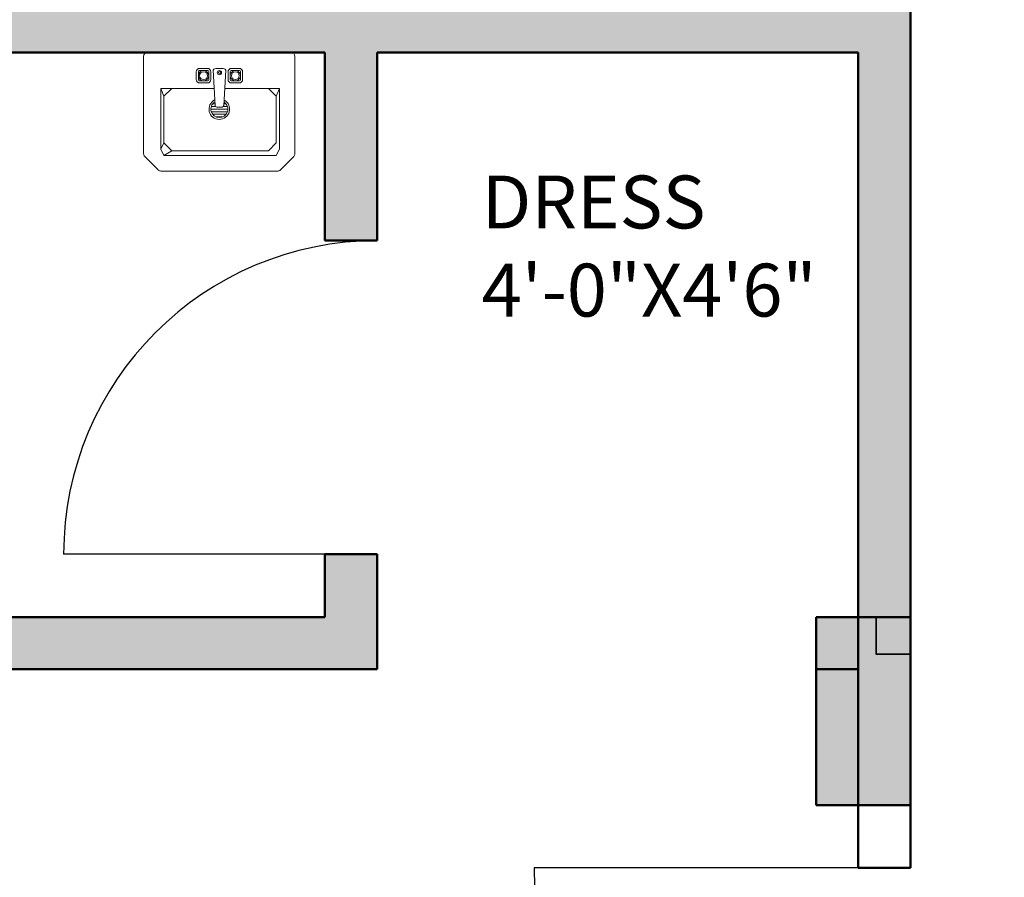
# Model space of a CAD drawing. Units: inches. Extents: x -7 to 1228, y -146 to 1091.
# Tile 73 of 88: x 722 to 816, y 703 to 785. Entities that reach past the tile are written whole.
import ezdxf

# ---------------------------------------------------------------- set-up
doc = ezdxf.new("R2010")
doc.units = ezdxf.units.IN
for name, color, linetype, lineweight in [('A-AREA-IDEN', 7, 'Continuous', 18), ('A-COLS', 6, 'Continuous', 35), ('A-DOOR', 4, 'Continuous', 25), ('A-FURN', 8, 'Continuous', 18), ('A-WALL', 7, 'Continuous', 50), ('A-WALL-PATT', 251, 'Continuous', 13)]:
    doc.layers.add(name, color=color, linetype=linetype, lineweight=lineweight)
doc.styles.get("Standard").update_dxf_attribs({"font": 'arial.ttf'})

# ---------------------------------------------------------------- blocks, each defined once
blk = doc.blocks.new('A$C4CB854FF')
for p, q in [((0.4725, 0.38), (0.0125, 0.38)), ((0, 0.3675), (0, 0.0552)), ((0.485, 0.0552), (0.485, 0.3675)), ((0.1677, 0.2932), (0.1677, 0.318)), ((0.1745, 0.2919), (0.1745, 0.3194)), ((0.1773, 0.3221), (0.2048, 0.3221)), ((0.1787, 0.329), (0.2034, 0.329)), ((0.2075, 0.3194), (0.2075, 0.2919)), ((0.2144, 0.318), (0.2144, 0.2932)), ((0.2279, 0.2104), (0.2213, 0.3235)), ((0.2337, 0.329), (0.2502, 0.329)), ((0.2625, 0.3235), (0.256, 0.2104)), ((0.2694, 0.318), (0.2694, 0.2932)), ((0.2763, 0.3194), (0.2763, 0.2919)), ((0.3065, 0.3221), (0.279, 0.3221)), ((0.3052, 0.329), (0.2804, 0.329)), ((0.3093, 0.2919), (0.3093, 0.3194)), ((0.3162, 0.2932), (0.3162, 0.318)), ((0.2048, 0.2891), (0.1773, 0.2891)), ((0.279, 0.2891), (0.3065, 0.2891)), ((0.05, 0.265), (0.2247, 0.265)), ((0.06, 0.24), (0.05, 0.265)), ((0.05, 0.07), (0.05, 0.265)), ((0.085, 0.265), (0.06, 0.24)), ((0.2034, 0.2822), (0.1787, 0.2822)), ((0.2591, 0.265), (0.43, 0.265)), ((0.2804, 0.2822), (0.3052, 0.2822)), ((0.395, 0.265), (0.42, 0.24)), ((0.42, 0.24), (0.43, 0.265)), ((0.43, 0.07), (0.43, 0.265)), ((0.06, 0.24), (0.06, 0.09)), ((0.42, 0.24), (0.42, 0.09)), ((0.2152, 0.1984), (0.2694, 0.1984)), ((0.2297, 0.2066), (0.2165, 0.2066)), ((0.2681, 0.1901), (0.2165, 0.1901)), ((0.2272, 0.2149), (0.2208, 0.2149)), ((0.2505, 0.2052), (0.2334, 0.2052)), ((0.2681, 0.2066), (0.2541, 0.2066)), ((0.2638, 0.2149), (0.2566, 0.2149)), ((0.2638, 0.1819), (0.2208, 0.1819)), ((0.2533, 0.1736), (0.2313, 0.1736)), ((0.05, 0.07), (0.06, 0.05)), ((0.06, 0.09), (0.085, 0.065)), ((0.085, 0.065), (0.395, 0.065)), ((0.42, 0.09), (0.395, 0.065)), ((0.395, 0.065), (0.42, 0.05)), ((0.42, 0.09), (0.43, 0.07)), ((0.43, 0.07), (0.42, 0.05)), ((0.0037, 0.0463), (0.0463, 0.0037)), ((0.42, 0.05), (0.06, 0.05)), ((0.4387, 0.0037), (0.4813, 0.0463)), ((0.0552, 0), (0.4298, 0))]:
    blk.add_line(p, q)
for centre, radius in [((0.191, 0.3056), 0.0165), ((0.191, 0.3056), 0.0127), ((0.2419, 0.3152), 0.00688), ((0.2419, 0.3152), 0.00344), ((0.2928, 0.3056), 0.0165), ((0.2928, 0.3056), 0.0127)]:
    blk.add_circle(centre, radius)
for centre, radius, start, end in [((0.0125, 0.3675), 0.0125, 90, 180), ((0.4725, 0.3675), 0.0125, 0, 90), ((0.1787, 0.318), 0.011, 90, 180), ((0.1773, 0.3194), 0.00275, 90, 180), ((0.2034, 0.318), 0.011, 0, 90), ((0.2048, 0.3194), 0.00275, 360, 90), ((0.2329, 0.314), 0.015, 87.1975, 140.7274), ((0.2509, 0.314), 0.015, 39.2726, 92.8025), ((0.2804, 0.318), 0.011, 90, 180), ((0.279, 0.3194), 0.00275, 90, 180), ((0.3052, 0.318), 0.011, 0, 90), ((0.3065, 0.3194), 0.00275, 360, 90), ((0.1787, 0.2932), 0.011, 180, 270), ((0.1773, 0.2919), 0.00275, 180, 270), ((0.2034, 0.2932), 0.011, 270, 0), ((0.2048, 0.2919), 0.00275, 270, 0), ((0.2804, 0.2932), 0.011, 180, 270), ((0.279, 0.2919), 0.00275, 180, 270), ((0.3052, 0.2932), 0.011, 270, 360), ((0.3065, 0.2919), 0.00275, 270, 0), ((0.2423, 0.1984), 0.033, 118.6883, 62.8686), ((0.2423, 0.1984), 0.0271, 124.7758, 57.2247), ((0.2334, 0.2107), 0.0055, 183.3274, 270), ((0.2505, 0.2107), 0.0055, 270, 356.6726), ((0.0125, 0.0552), 0.0125, 180, 225), ((0.4725, 0.0552), 0.0125, 315, 0), ((0.0552, 0.0125), 0.0125, 225, 270), ((0.4298, 0.0125), 0.0125, 270, 315)]:
    blk.add_arc(centre, radius, start, end)
blk = doc.blocks.new('DOOR-750')
blk.add_line((30, 30), (30, 0))
blk.add_arc((30, 30), 30, 180, 270)
blk = doc.blocks.new('DOOR-900')
blk.add_line((36, 0), (36, 36))
blk.add_arc((36, 0), 36, 90, 180)

msp = doc.modelspace()

# ---------------------------------------------------------------- hatches: boundary and pattern name
at = {"layer": 'A-COLS'}
h = msp.add_hatch(color=256, dxfattribs=at)
h.dxf.hatch_style = 1
h.paths.add_polyline_path([(807, 724.454), (803.711, 724.454), (803.711, 728), (798, 728), (798, 710), (807, 710)])
h = msp.add_hatch(color=256, dxfattribs=at)
h.dxf.hatch_style = 1
h.paths.add_polyline_path([(807, 724.454), (807, 728), (803.711, 728), (803.711, 724.454)])
at = {"layer": 'A-WALL-PATT'}
h = msp.add_hatch(color=256, dxfattribs=at)
h.dxf.hatch_style = 1
h.paths.add_polyline_path([(69, 568), (60, 568), (60, 493), (63.289, 493), (69, 493)])
h.paths.add_polyline_path([(69, 662.405), (60, 662.405), (60, 586), (69, 586)], flags=17)
h.paths.add_polyline_path([(69, 723), (184, 723), (184, 734), (179, 734), (179, 728), (69, 728), (69, 741.623), (60, 741.623), (60, 698.405), (69, 698.405)], flags=17)
h.paths.add_polyline_path([(69, 782), (231, 782), (231, 728), (231, 723), (231, 586), (236, 586), (236, 787), (69, 787), (69, 800.126), (60, 800.126), (60, 765.623), (69, 765.623)])
h.paths.add_polyline_path([(184, 842), (189, 842), (189, 848), (173, 848), (173, 842), (179, 842), (179, 787), (184, 787)])
h.paths.add_polyline_path([(118.22, 69), (69, 69), (69, 60), (118.22, 60)])
h.paths.add_polyline_path([(227, 69), (154.22, 69), (154.22, 60), (227, 60)])
h.paths.add_polyline_path([(236, 60), (232.711, 60), (227, 60), (227, 36), (236, 36)])
h.paths.add_polyline_path([(389, 60), (380, 60), (380, 36), (389, 36)])
h.paths.add_polyline_path([(384, 181), (380, 181), (380, 115), (380, 78), (384, 78)])
h.paths.add_polyline_path([(380, 115), (334.547, 115), (334.547, 109), (380, 109)])
h.paths.add_polyline_path([(274.547, 115), (236, 115), (236, 201), (232.711, 201), (231, 201), (231, 78), (236, 78), (236, 109), (274.547, 109)])
h.paths.add_polyline_path([(69, 123), (60, 123), (60, 78), (69, 78)])
h.paths.add_polyline_path([(69, 201), (60, 201), (60, 159), (69, 159)])
h.paths.add_polyline_path([(143, 219), (69, 219), (69, 213), (143, 213)], flags=17)
h.paths.add_polyline_path([(189, 219), (184, 219), (184, 274), (231, 274), (231, 219), (236, 219), (236, 279), (184, 279), (184, 297), (179, 297), (179, 279), (69, 279), (69, 290.912), (60, 290.912), (60, 262.179), (69, 262.179), (69, 274), (179, 274), (179, 219), (173, 219), (173, 213), (189, 213)])
h.paths.add_polyline_path([(69, 238.179), (60, 238.179), (60, 219), (69, 219)], flags=17)
h.paths.add_polyline_path([(69, 333), (60, 333), (60, 314.912), (69, 314.912), (69, 316.965)])
h.paths.add_polyline_path([(190, 338), (184, 338), (69, 338), (69, 333), (179, 333), (179, 327), (184, 327), (184, 333.021), (190, 333.046)])
h.paths.add_polyline_path([(69, 386.806), (60, 386.806), (60, 351), (69, 351)])
h.paths.add_polyline_path([(69, 475), (60, 475), (60, 422.806), (69, 422.806)])
h.paths.add_polyline_path([(236, 475), (231, 475), (231, 351.238), (236, 351.238)])
h.paths.add_polyline_path([(384, 475), (380, 475), (380, 362), (384, 362)])
h.paths.add_polyline_path([(547, 307), (439, 307), (439, 356), (445, 356), (445, 362), (433, 362), (433, 307), (380, 307), (380, 244), (380, 241), (384, 241), (384, 301), (433, 301), (433, 277), (439, 277), (439, 301), (547, 301)])
h.paths.add_polyline_path([(547, 241), (439, 241), (439, 247), (433, 247), (433, 235), (547, 235)])
h.paths.add_polyline_path([(450, 69), (440.286, 69), (424.889, 69), (389, 69), (389, 60), (450, 60)])
h.paths.add_polyline_path([(547, 69), (486, 69), (486, 60), (547, 60)])
h.paths.add_polyline_path([(556, 148.268), (547, 148.268), (547, 78), (556, 78)])
h.paths.add_polyline_path([(556, 223), (547, 223), (547, 195), (547, 184.268), (556, 184.268)])
h.paths.add_polyline_path([(556, 311.192), (547, 311.192), (547, 273.075), (556, 273.075)])
h.paths.add_polyline_path([(556, 344), (552.711, 344), (547, 344), (547, 335.192), (556, 335.192)])
h.paths.add_polyline_path([(556, 249.075), (547, 249.075), (547, 241), (556, 241)])
h.paths.add_polyline_path([(547, 362), (475, 362), (475, 356), (547, 356)], flags=0)
h.paths.add_polyline_path([(556, 399.621), (547, 399.621), (547, 362), (556, 362)])
h.paths.add_polyline_path([(556, 475), (547, 475), (547, 435.621), (556, 435.621)])
h.paths.add_polyline_path([(547, 493), (389, 493), (389, 487), (547, 487)])
h.paths.add_polyline_path([(380, 493), (278, 493), (278, 487), (380, 487)])
h.paths.add_polyline_path([(227, 493), (69, 493), (69, 487), (227, 487)])
h.paths.add_polyline_path([(643, 122.445), (634, 122.445), (634, 78), (643, 78)])
h.paths.add_polyline_path([(702.5, 69), (692.786, 69), (677.389, 69), (643, 69), (643, 60), (702.5, 60)])
h.paths.add_polyline_path([(798, 69), (738.5, 69), (738.5, 60), (798, 60)])
h.paths.add_polyline_path([(807, 60), (803.711, 60), (798, 60), (798, 36), (807, 36)])
h.paths.add_polyline_path([(807, 109), (846.751, 109), (846.751, 115), (807, 115), (807, 159), (802, 159), (802, 78), (807, 78)])
h.paths.add_polyline_path([(807, 201), (802, 201), (802, 195), (807, 195)])
h.paths.add_polyline_path([(643, 201), (634, 201), (634, 158.445), (643, 158.445)])
h.paths.add_polyline_path([(756, 225), (751, 225), (751, 219), (643, 219), (643, 213), (756, 213)])
h.paths.add_polyline_path([(643, 240.848), (634, 240.848), (634, 219), (643, 219)])
h.paths.add_polyline_path([(643, 274), (643, 288.629), (634, 288.629), (634, 264.848), (643, 264.848)])
h.paths.add_polyline_path([(802, 279), (756, 279), (756, 297), (751, 297), (751, 279), (643, 279), (643, 274), (751, 274), (751, 255), (756, 255), (756, 274), (802, 274)])
h.paths.add_polyline_path([(807, 333), (803.711, 333), (802, 333), (802, 279), (802, 274), (802, 219), (807, 219)])
h.paths.add_polyline_path([(956, 182), (951, 182), (951, 115), (906.751, 115), (906.751, 109), (951, 109), (951, 78), (956, 78)])
h.paths.add_polyline_path([(960, 60), (951, 60), (951, 36), (960, 36)])
h.paths.add_polyline_path([(1021, 69), (1005.781, 69), (960, 69), (960, 60), (1021, 60)])
h.paths.add_polyline_path([(956, 224), (951, 224), (951, 218), (956, 218)])
h.paths.add_polyline_path([(956, 302), (1004, 302), (1004, 278), (1010, 278), (1010, 302), (1118, 302), (1118, 290.809), (1127, 290.809), (1127, 326.968), (1118, 326.968), (1118, 320.966), (1118, 307), (1010, 307), (1010, 356), (1016, 356), (1016, 362), (1004, 362), (1004, 307), (951, 307), (951, 244), (951, 242), (954.289, 242), (956, 242)])
h.paths.add_polyline_path([(643, 333), (634, 333), (634, 312.629), (643, 312.629), (643, 316.965)])
h.paths.add_polyline_path([(756, 338), (643, 338), (643, 333), (751, 333), (751, 327), (756, 327)])
h.paths.add_polyline_path([(643, 388), (634, 388), (634, 351), (643, 351)])
h.paths.add_polyline_path([(807, 357), (802, 357), (802, 351), (807, 351)])
h.paths.add_polyline_path([(807, 475), (802, 475), (802, 393), (807, 393)])
h.paths.add_polyline_path([(643, 475), (634, 475), (634, 424), (643, 424)])
h.paths.add_polyline_path([(798, 493), (643, 493), (643, 487), (798, 487)])
h.paths.add_polyline_path([(634, 493), (556, 493), (556, 487), (634, 487)])
h.paths.add_polyline_path([(813, 493), (807, 493), (807, 487), (813, 487)])
h.paths.add_polyline_path([(951, 493), (849, 493), (849, 487), (951, 487)])
h.paths.add_polyline_path([(956, 484), (951, 484), (951, 374), (956, 374)])
h.paths.add_polyline_path([(1109, 493), (969, 493), (969, 487), (1109, 487)])
h.paths.add_polyline_path([(1127, 484), (1118, 484), (1118, 450.641), (1127, 450.641)])
h.paths.add_polyline_path([(1127, 414.641), (1118, 414.641), (1118, 365), (1127, 365)])
h.paths.add_polyline_path([(1109, 362), (1046, 362), (1046, 356), (1109, 356)], flags=17)
h.paths.add_polyline_path([(1127, 356), (1123.454, 356), (1118, 356), (1118, 350.968), (1127, 350.968)], flags=0)
h.paths.add_polyline_path([(1127, 266.809), (1118, 266.809), (1118, 262.361), (1118, 242), (1127, 242)], flags=17)
h.paths.add_polyline_path([(1118, 242), (1010, 242), (1010, 248), (1004, 248), (1004, 237), (1118, 237)])
h.paths.add_polyline_path([(1127, 224), (1118, 224), (1118, 170), (1127, 170)])
h.paths.add_polyline_path([(1127, 134), (1118, 134), (1118, 78), (1127, 78)])
h.paths.add_polyline_path([(1118, 69), (1057, 69), (1057, 60), (1118, 60)])
h.paths.add_polyline_path([(227, 571.546), (227, 574), (69, 574), (69, 568), (227, 568)])
h.paths.add_polyline_path([(380, 571.546), (380, 574), (278, 574), (278, 568), (380, 568)])
h.paths.add_polyline_path([(242, 574), (236, 574), (236, 568), (242, 568)])
h.paths.add_polyline_path([(547, 571.546), (547, 574), (389, 574), (389, 568), (547, 568)])
h.paths.add_polyline_path([(384, 733), (380, 733), (380, 586), (384, 586)])
h.paths.add_polyline_path([(556, 646), (634, 646), (634, 655), (547, 655), (547, 586), (556, 586)])
h.paths.add_polyline_path([(634, 574), (556, 574), (556, 568), (634, 568)])
h.paths.add_polyline_path([(643, 655), (634, 655), (634, 586), (643, 586)])
h.paths.add_polyline_path([(798, 574), (643, 574), (643, 568), (798, 568)])
h.paths.add_polyline_path([(643, 663.854), (634, 663.854), (634, 655), (643, 655)])
h.paths.add_polyline_path([(556, 676.967), (547, 676.967), (547, 655), (556, 655)])
h.paths.add_polyline_path([(556, 733), (547, 733), (547, 712.967), (556, 712.967)])
h.paths.add_polyline_path([(643, 710), (634, 710), (634, 699.854), (643, 699.854)])
h.paths.add_polyline_path([(807, 668), (802, 668), (802, 586), (807, 586)])
h.paths.add_polyline_path([(951, 574), (849, 574), (849, 568), (951, 568)])
h.paths.add_polyline_path([(956, 691), (951, 691), (951, 577), (956, 577)])
h.paths.add_polyline_path([(1109, 574), (969, 574), (969, 568), (1109, 568)])
h.paths.add_polyline_path([(1127, 643.403), (1118, 643.403), (1118, 577), (1127, 577)])
h.paths.add_polyline_path([(1127, 568), (1123.454, 568), (1118, 568), (1118, 493), (1127, 493)])
h.paths.add_polyline_path([(1127, 733), (1118, 733), (1118, 679.403), (1127, 679.403)])
h.paths.add_polyline_path([(1127, 777.348), (1118, 777.348), (1118, 770.035), (1118, 751), (1127, 751)], flags=17)
h.paths.add_polyline_path([(1118, 751), (1010, 751), (1010, 757), (1004, 757), (1004, 745), (1118, 745)])
h.paths.add_polyline_path([(956, 811), (1004, 811), (1004, 787), (1010, 787), (1010, 811), (1017.874, 811), (1017.874, 811.627, -0.414214), (1018.247, 812), (1031.978, 812, -0.414214), (1032.351, 811.627), (1032.351, 811), (1118, 811), (1118, 801.348), (1127, 801.348), (1127, 834.685), (1118, 834.685), (1118, 830.238), (1118, 817), (1010, 817), (1010, 866), (1016, 866), (1016, 872), (1004, 872), (1004, 817), (956, 817), (956, 866), (951, 866), (951, 751), (954.289, 751), (956, 751)])
h.paths.add_polyline_path([(1118, 872), (1046, 872), (1046, 866), (1118, 866)], flags=17)
h.paths.add_polyline_path([(1127, 924.711), (1118, 924.711), (1118, 884), (1127, 884)])
h.paths.add_polyline_path([(1127, 866), (1123.711, 866), (1118, 866), (1118, 858.685), (1127, 858.685)], flags=17)
h.paths.add_polyline_path([(956, 983), (951, 983), (951, 952), (807, 952), (807, 983), (802, 983), (802, 902), (807, 902), (807, 946), (951, 946), (951, 884), (956, 884)])
h.paths.add_polyline_path([(807, 842), (802, 842), (802, 787), (756, 787), (756, 806), (751, 806), (751, 787), (643, 787), (643, 782), (751, 782), (751, 764), (756, 764), (756, 782), (802, 782), (802, 728), (807, 728)])
h.paths.add_polyline_path([(756, 848), (643, 848), (643, 842), (751, 842), (751, 836), (756, 836)])
h.paths.add_polyline_path([(756, 734), (751, 734), (751, 728), (643, 728), (643, 723), (756, 723)])
h.paths.add_polyline_path([(643, 749.791), (634, 749.791), (634, 728), (637.289, 728), (643, 728)])
h.paths.add_polyline_path([(643, 805.405), (634, 805.405), (634, 773.791), (643, 773.791)])
h.paths.add_polyline_path([(643, 896.663), (634, 896.663), (634, 860), (637.289, 860), (643, 860)])
h.paths.add_polyline_path([(643, 842), (634, 842), (634, 829.405), (643, 829.405)])
h.paths.add_polyline_path([(643, 983), (634, 983), (634, 932.663), (643, 932.663)])
h.paths.add_polyline_path([(1127, 983), (1118, 983), (1118, 960.711), (1127, 960.711)])
h.paths.add_polyline_path([(1118, 1001), (1077.525, 1001), (1077.525, 992), (1118, 992)])
h.paths.add_polyline_path([(1041.525, 1001), (960, 1001), (960, 992), (1041.525, 992)])
h.paths.add_polyline_path([(960, 1025), (951, 1025), (951, 1001), (954.289, 1001), (960, 1001)])
h.paths.add_polyline_path([(807, 1025), (798, 1025), (798, 1001), (807, 1001)])
h.paths.add_polyline_path([(798, 1001), (738.5, 1001), (738.5, 992), (798, 992)])
h.paths.add_polyline_path([(702.5, 1001), (643, 1001), (643, 992), (702.5, 992)])
h.paths.add_polyline_path([(547, 1001), (499.113, 1001), (499.113, 992), (547, 992)])
h.paths.add_polyline_path([(463.113, 1001), (389, 1001), (389, 992), (463.113, 992)])
h.paths.add_polyline_path([(389, 1025), (380, 1025), (380, 1022), (380, 1001), (383.289, 1001), (389, 1001)])
h.paths.add_polyline_path([(236, 1025), (227, 1025), (227, 1001), (236, 1001)])
h.paths.add_polyline_path([(236, 983), (231, 983), (231, 860), (236, 860)])
h.paths.add_polyline_path([(274.547, 952), (236, 952), (236, 946), (274.547, 946)])
h.paths.add_polyline_path([(380, 952), (334.547, 952), (334.547, 946), (380, 946)])
h.paths.add_polyline_path([(384, 983), (380, 983), (380, 884), (383.289, 884), (384, 884)])
h.paths.add_polyline_path([(227, 1001), (155.012, 1001), (155.012, 992), (162.875, 992), (227, 992)])
h.paths.add_polyline_path([(119.012, 1001), (69, 1001), (69, 992), (119.012, 992)])
h.paths.add_polyline_path([(69, 983), (60, 983), (60, 922.987), (69, 922.987)])
h.paths.add_polyline_path([(69, 886.987), (60, 886.987), (60, 860), (63.289, 860), (69, 860)])
h.paths.add_polyline_path([(143, 848), (69, 848), (69, 842), (143, 842)])

# ---------------------------------------------------------------- linework, layer by layer
at = {"layer": 'A-COLS'}
msp.add_lwpolyline([(807, 728), (803.711, 728), (803.711, 724.454), (807, 724.454)], close=True, dxfattribs=at)
at = {"layer": 'A-WALL'}
for p, q in [((807, 866), (807, 704)), ((807, 704), (807, 866)), ((751, 782), (643, 782)), ((751, 782), (751, 764)), ((802, 782), (756, 782)), ((756, 782), (756, 764)), ((802, 782), (802, 728)), ((802, 704), (802, 782)), ((756, 764), (751, 764)), ((756, 734), (751, 734)), ((751, 734), (751, 728)), ((756, 734), (756, 723)), ((751, 728), (643, 728)), ((802, 728), (798, 728)), ((807, 728), (798, 728)), ((798, 728), (798, 710)), ((807, 710), (807, 728)), ((756, 723), (643, 723)), ((802, 723), (798, 723)), ((802, 723), (802, 704)), ((798, 710), (807, 710)), ((807, 704), (802, 704))]:
    msp.add_line(p, q, dxfattribs=at)

# ---------------------------------------------------------------- block references
at = {"layer": 'A-DOOR'}
for name, p, rotation in [('DOOR-750', (726, 764), 270), ('DOOR-900', (807, 668), 89.99999999999964)]:
    msp.add_blockref(name, p, dxfattribs=dict(at, rotation=rotation))
at = {"layer": 'A-FURN', "xscale": -29.84864686937646, "yscale": 29.84864686937646, "zscale": 29.84864686937646}
msp.add_blockref('A$C4CB854FF', (748.128, 770.658), dxfattribs=at)

# ---------------------------------------------------------------- texts
at = {"layer": 'A-AREA-IDEN', "insert": (765.993, 770.226), "char_height": 5.0568, "attachment_point": 1}
msp.add_mtext_dynamic_manual_height_columns('DRESS\\P4\'-0"X4\'6"', width=137.28212, gutter_width=25.284, heights=[0], dxfattribs=at)

doc.saveas('drawing.dxf')
